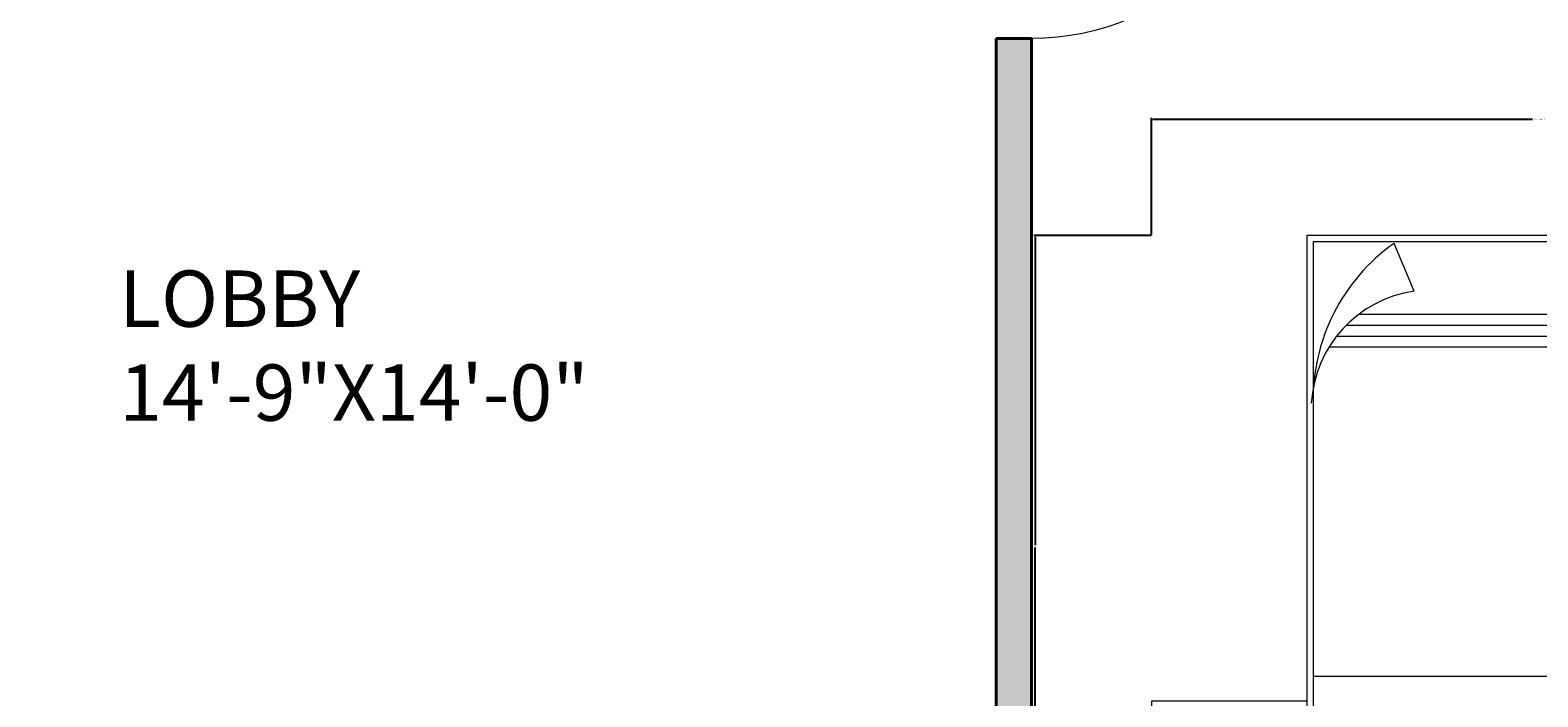
# Model space of a CAD drawing. Units: inches. Extents: x 2330 to 3943, y 1763 to 3461.
# Tile 21 of 40: x 3018 to 3231, y 2734 to 2829. Entities that reach past the tile are written whole.
import ezdxf

# ---------------------------------------------------------------- set-up
doc = ezdxf.new("R2010")
doc.units = ezdxf.units.IN
for name, color, linetype, lineweight in [('A-ANNO-DIMS', 2, 'Continuous', 18), ('A-AREA-IDEN', 7, 'Continuous', 18), ('A-DOOR', 4, 'Continuous', 18), ('A-FURN', 8, 'Continuous', 13), ('A-WALL', 7, 'Continuous', 40), ('A-WALL-PATT', 252, 'Continuous', 13)]:
    doc.layers.add(name, color=color, linetype=linetype, lineweight=lineweight)
doc.styles.get("Standard").update_dxf_attribs({"font": 'arial.ttf'})
doc.dimstyles.get("Standard").update_dxf_attribs({"dimtxt": 0.18, "dimasz": 0.18, "dimexe": 0.18, "dimexo": 0.0625, "dimgap": 0.09, "dimtad": 0, "dimtih": 1, "dimtoh": 1, "dimdec": 4, "dimzin": 0, "dimdsep": 46, "dimtxsty": 'Standard', "dimcen": 0.09, "dimadec": 0, "dimazin": 0, "dimtfac": 1, "dimtdec": 4, "dimtofl": 0, "dimtmove": 0, "dimatfit": 3, "dimfxl": 1, "dimtolj": 1, "dimtzin": 0, "dimarcsym": 0})

# ---------------------------------------------------------------- blocks, each defined once
blk = doc.blocks.new('A$C057D194F')
for p, q in [((0, 1.5, -0.1688), (0, 2, -0.1688)), ((0, 2, -0.1688), (0.5, 2, -0.1688)), ((0.5, 2, -0.1688), (0.5, 0, -0.1688)), ((2, 2, -0.1688), (0.5, 2, -0.1688)), ((2, 0, -0.1688), (2, 2, -0.1688)), ((2.5, 2, -0.1688), (2, 2, -0.1688)), ((2.5, 1.5, -0.1688), (2.5, 2, -0.1688)), ((1.98, 1.98, -0.1688), (0.52, 1.98, -0.1688)), ((0.52, 1.98, -0.1688), (0.52, 0.02, -0.1688)), ((1.0907, 1.9539, -0.1688), (0.7735, 1.9539, -0.1688)), ((1.8224, 1.9539, -0.1688), (1.5052, 1.9539, -0.1688)), ((1.98, 0.02, -0.1688), (1.98, 1.98, -0.1688)), ((0.2687, 1.9081, -0.1688), (0.2687, 1.761, -0.1688)), ((0.2687, 1.6081, -0.1688), (0.2687, 1.9081, -0.1688)), ((1.0907, 1.9339, -0.1688), (0.7735, 1.9339, -0.1688)), ((1.8224, 1.9339, -0.1688), (1.5052, 1.9339, -0.1688)), ((2.2313, 1.9081, -0.1688), (2.2313, 1.761, -0.1688)), ((2.2313, 1.6081, -0.1688), (2.2313, 1.9081, -0.1688)), ((0.6935, 1.8739, -0.1688), (0.6935, 1.7322, -0.1688)), ((0.7135, 1.8739, -0.1688), (0.7135, 1.7322, -0.1688)), ((1.1507, 1.7322, -0.1688), (1.1507, 1.8739, -0.1688)), ((1.1707, 1.7322, -0.1688), (1.1707, 1.8739, -0.1688)), ((1.4252, 1.8739, -0.1688), (1.4252, 1.7322, -0.1688)), ((1.4452, 1.8739, -0.1688), (1.4452, 1.7322, -0.1688)), ((1.8824, 1.7322, -0.1688), (1.8824, 1.8739, -0.1688)), ((1.9024, 1.7322, -0.1688), (1.9024, 1.8739, -0.1688)), ((0.4194, 1.761, -0.1688), (0.1194, 1.761, -0.1688)), ((0.2687, 1.761, -0.1688), (0.4194, 1.761, -0.1688)), ((0.2687, 1.761, -0.1688), (0.2687, 1.6081, -0.1688)), ((2.0806, 1.761, -0.1688), (2.3806, 1.761, -0.1688)), ((2.2313, 1.761, -0.1688), (2.0806, 1.761, -0.1688)), ((2.2313, 1.761, -0.1688), (2.2313, 1.6081, -0.1688)), ((0.7735, 1.6722, -0.1688), (1.0907, 1.6722, -0.1688)), ((0.7735, 1.6522, -0.1688), (1.0907, 1.6522, -0.1688)), ((1.5052, 1.6722, -0.1688), (1.8224, 1.6722, -0.1688)), ((1.5052, 1.6522, -0.1688), (1.8224, 1.6522, -0.1688)), ((1.98, 1.5693, -0.1688), (0.52, 1.5693, -0.1688)), ((0.5, 1.5, -0.1688), (0, 1.5, -0.1688)), ((2, 1.5, -0.1688), (2.5, 1.5, -0.1688)), ((1.98, 1.4193, -0.1688), (0.52, 1.4193, -0.1688)), ((0.6969, 0.02, -0.1688), (0.6969, 1.4193, -0.1688)), ((0.7319, 0.02, -0.1688), (0.7319, 1.4193, -0.1688)), ((0.7669, 0.02, -0.1688), (0.7669, 1.4193, -0.1688)), ((0.8019, 0.02, -0.1688), (0.8019, 1.4193, -0.1688)), ((0.52, 0.3595, -0.1688), (1.9292, 0.3595, -0.1688)), ((0.52, 0.3245, -0.1688), (1.905, 0.3245, -0.1688)), ((0.52, 0.2895, -0.1688), (1.8742, 0.2895, -0.1688)), ((0.52, 0.2545, -0.1688), (1.8344, 0.2545, -0.1688)), ((1.6548, 0.1789, -0.1688), (1.7198, 0.0251, -0.1688)), ((0.52, 0.02, -0.1688), (1.98, 0.02, -0.1688)), ((0.5, 0, -0.1688), (2, 0, -0.1688))]:
    blk.add_line(p, q)
for centre, radius, start, end in [((0.7735, 1.8739, -0.1688), 0.08, 90, 180), ((1.0907, 1.8739, -0.1688), 0.08, 0, 90), ((1.5052, 1.8739, -0.1688), 0.08, 90, 180), ((1.8224, 1.8739, -0.1688), 0.08, 0, 90), ((0.7735, 1.8739, -0.1688), 0.06, 90, 180), ((1.0907, 1.8739, -0.1688), 0.06, 0, 90), ((1.5052, 1.8739, -0.1688), 0.06, 90, 180), ((1.8224, 1.8739, -0.1688), 0.06, 0, 90), ((0.7735, 1.7322, -0.1688), 0.08, 180, 270), ((0.7735, 1.7322, -0.1688), 0.06, 180, 270), ((1.0907, 1.7322, -0.1688), 0.08, 270, 0), ((1.0907, 1.7322, -0.1688), 0.06, 270, 0), ((1.5052, 1.7322, -0.1688), 0.08, 180, 270), ((1.5052, 1.7322, -0.1688), 0.06, 180, 270), ((1.8224, 1.7322, -0.1688), 0.08, 270, 0), ((1.8224, 1.7322, -0.1688), 0.06, 270, 0), ((1.5992, 0.5623, -0.1688), 0.3874, 278.2518, 356.6808), ((1.363, 0.5286, -0.1688), 0.6171, 305.3295, 1.0459)]:
    blk.add_arc(centre, radius, start, end)
blk.add_ellipse((0.2687, 1.761, -0.1688), major_axis=(0, -0.1351), ratio=0.975448)
at = {"extrusion": (0, 0, -1)}
blk.add_ellipse((2.2313, 1.761, -0.1688), major_axis=(0, 0.1351), ratio=0.975448, dxfattribs=at)
for p in [(0.2687, 1.761, -0.1688), (2.2313, 1.761, -0.1688)]:
    blk.add_point(p)
blk = doc.blocks.new('DOOR-SINGLE-36IN')
blk.add_line((0, 0), (-36, 0))
blk.add_arc((0, 0), 36, 180, 270)
blk = doc.blocks.new('*D57')
at = {"layer": 'A-ANNO-DIMS', "color": 0, "lineweight": -2, "transparency": 16777216}
for p, q in [((3176.71, 2799.74), (3176.71, 2816.38)), ((3286.9, 2799.74), (3286.9, 2816.38)), ((3176.89, 2816.2), (3230.73, 2816.2)), ((3286.72, 2816.2), (3232.88, 2816.2))]:
    blk.add_line(p, q, dxfattribs=at)
at = {"layer": 'A-ANNO-DIMS', "color": 0, "transparency": 16777216}
for points in [[(3176.89, 2816.23), (3176.89, 2816.17), (3176.71, 2816.2)], [(3286.72, 2816.23), (3286.72, 2816.17), (3286.9, 2816.2)]]:
    blk.add_solid(points, dxfattribs=at)
at = {"layer": 'Defpoints', "color": 0, "transparency": 16777216}
for p in [(3176.71, 2816.2), (3176.71, 2799.68), (3286.9, 2799.68)]:
    blk.add_point(p, dxfattribs=at)
at = {"layer": 'A-ANNO-DIMS', "color": 0, "transparency": 16777216, "insert": (3231.8, 2816.2), "char_height": 0.18, "attachment_point": 5}
blk.add_mtext('\\A1;SINGLE BED 110', dxfattribs=at)
blk = doc.blocks.new('*D58')
at = {"layer": 'A-ANNO-DIMS', "color": 0, "lineweight": -2, "transparency": 16777216}
for p, q in [((3176.65, 2799.68), (3160, 2799.68)), ((3160.18, 2799.5), (3160.18, 2755.78)), ((3160.18, 2711.71), (3160.18, 2755.42)), ((3176.65, 2711.53), (3160, 2711.53))]:
    blk.add_line(p, q, dxfattribs=at)
at = {"layer": 'A-ANNO-DIMS', "color": 0, "transparency": 16777216}
for points in [[(3160.15, 2799.5), (3160.21, 2799.5), (3160.18, 2799.68)], [(3160.15, 2711.71), (3160.21, 2711.71), (3160.18, 2711.53)]]:
    blk.add_solid(points, dxfattribs=at)
at = {"layer": 'Defpoints', "color": 0, "transparency": 16777216}
for p in [(3176.71, 2799.68), (3160.18, 2711.53), (3176.71, 2711.53)]:
    blk.add_point(p, dxfattribs=at)
at = {"layer": 'A-ANNO-DIMS', "color": 0, "transparency": 16777216, "insert": (3160.18, 2755.6), "char_height": 0.18, "attachment_point": 5}
blk.add_mtext('\\A1;88', dxfattribs=at)
blk = doc.blocks.new('*D96')
at = {"layer": 'A-ANNO-DIMS', "color": 0, "lineweight": -2, "transparency": 16777216}
for p, q in [((3604.65, 2753.34), (3417.72, 2743.73)), ((3105.6, 2727.69), (3105.78, 2727.69)), ((3105.69, 2727.6), (3105.69, 2727.78))]:
    blk.add_line(p, q, dxfattribs=at)
at = {"layer": 'A-ANNO-DIMS', "color": 0, "transparency": 16777216}
blk.add_solid([(3417.72, 2743.76), (3417.72, 2743.7), (3417.54, 2743.72)], dxfattribs=at)
at = {"layer": 'Defpoints', "color": 0, "transparency": 16777216}
for p in [(3417.54, 2743.72), (3105.69, 2727.69)]:
    blk.add_point(p, dxfattribs=at)
at = {"layer": 'A-ANNO-DIMS', "color": 0, "transparency": 16777216, "insert": (3605.39, 2753.34), "char_height": 0.18, "attachment_point": 5}
blk.add_mtext('\\A1;2X R312.26', dxfattribs=at)

msp = doc.modelspace()

# ---------------------------------------------------------------- hatches: boundary and pattern name
at = {"layer": 'A-WALL-PATT'}
h = msp.add_hatch(color=256, dxfattribs=at)
h.dxf.hatch_style = 1
h.paths.add_polyline_path([(3420.6832, 2705.6524), (3159.6605, 2705.6524), (3159.6605, 2827.6524), (3154.6605, 2827.6524), (3154.6605, 2705.6524), (3017.6605, 2705.6524), (3017.6605, 2700.6524), (3238.6605, 2700.6524), (3238.6605, 2605.6524), (3247.6605, 2605.6524), (3247.6605, 2610.6524), (3243.6605, 2610.6524), (3243.6605, 2700.6524), (3411.2593, 2700.6524, -0.02528333), (3406.9698, 2669.9468), (3415.809, 2668.2528, 0.02988796)])

# ---------------------------------------------------------------- linework, layer by layer
at = {"layer": 'A-WALL'}
for p, q in [((3154.6605, 2827.6524), (3159.6605, 2827.6524)), ((3154.6605, 2827.6524), (3154.6605, 2705.6524)), ((3159.6605, 2827.6524), (3159.6605, 2705.6524))]:
    msp.add_line(p, q, dxfattribs=at)

# ---------------------------------------------------------------- block references
at = {"layer": 'A-DOOR', "extrusion": (0, 0, -1), "zscale": -1}
msp.add_blockref('DOOR-SINGLE-36IN', (-3159.6605, 2863.6524), dxfattribs=at)
at = {"layer": 'A-FURN', "xscale": 44.07393684478161, "yscale": 44.07393684478161, "zscale": 44.07393684478161, "rotation": 180}
msp.add_blockref('A$C057D194F', (3286.8969, 2799.6765, 7.4375), dxfattribs=at)

# ---------------------------------------------------------------- texts
at = {"layer": 'A-AREA-IDEN', "insert": (3030.2959, 2794.7224), "char_height": 8, "attachment_point": 1}
msp.add_mtext_dynamic_manual_height_columns('LOBBY\\P14\'-9"X14\'-0"', width=89.990069, gutter_width=12.5, heights=[0], dxfattribs=at)

# ---------------------------------------------------------------- dimensions: what is measured, and where the dimension line sits
at = {"layer": 'A-ANNO-DIMS'}
dim = msp.add_linear_dim(base=(3176.7121, 2816.2042), p1=(3286.8969, 2799.6765), p2=(3176.7121, 2799.6765), angle=180, text='SINGLE BED <>', dimstyle='Standard', override={"dimdec": 0, "dimlfac": 1, "dimrnd": 0, "dimzin": 0, "dimdsep": 46, "dimlunit": 2}, dxfattribs=at)
dim.commit()
dim.dimension.update_dxf_attribs({"geometry": '*D57', "text_midpoint": (3231.8045, 2816.2042)})
dim = msp.add_linear_dim(base=(3160.1844, 2711.5286), p1=(3176.7121, 2799.6765), p2=(3176.7121, 2711.5286), angle=270, dimstyle='Standard', override={"dimdec": 0, "dimlfac": 1, "dimrnd": 0, "dimzin": 0, "dimdsep": 46, "dimlunit": 2}, dxfattribs=at)
dim.commit()
dim.dimension.update_dxf_attribs({"geometry": '*D58', "text_midpoint": (3160.1844, 2755.6026)})
dim = msp.add_radius_dim(center=(3105.6935, 2727.6869), mpoint=(3417.5409, 2743.723), text='2X <>', dimstyle='Standard', override={"dimdec": 2, "dimlfac": 1, "dimrnd": 0, "dimzin": 0, "dimdsep": 46, "dimlunit": 2}, dxfattribs=at)
dim.commit()
dim.dimension.update_dxf_attribs({"geometry": '*D96', "text_midpoint": (3604.6494, 2753.3446), "dimtype": 164})

doc.saveas('drawing.dxf')
